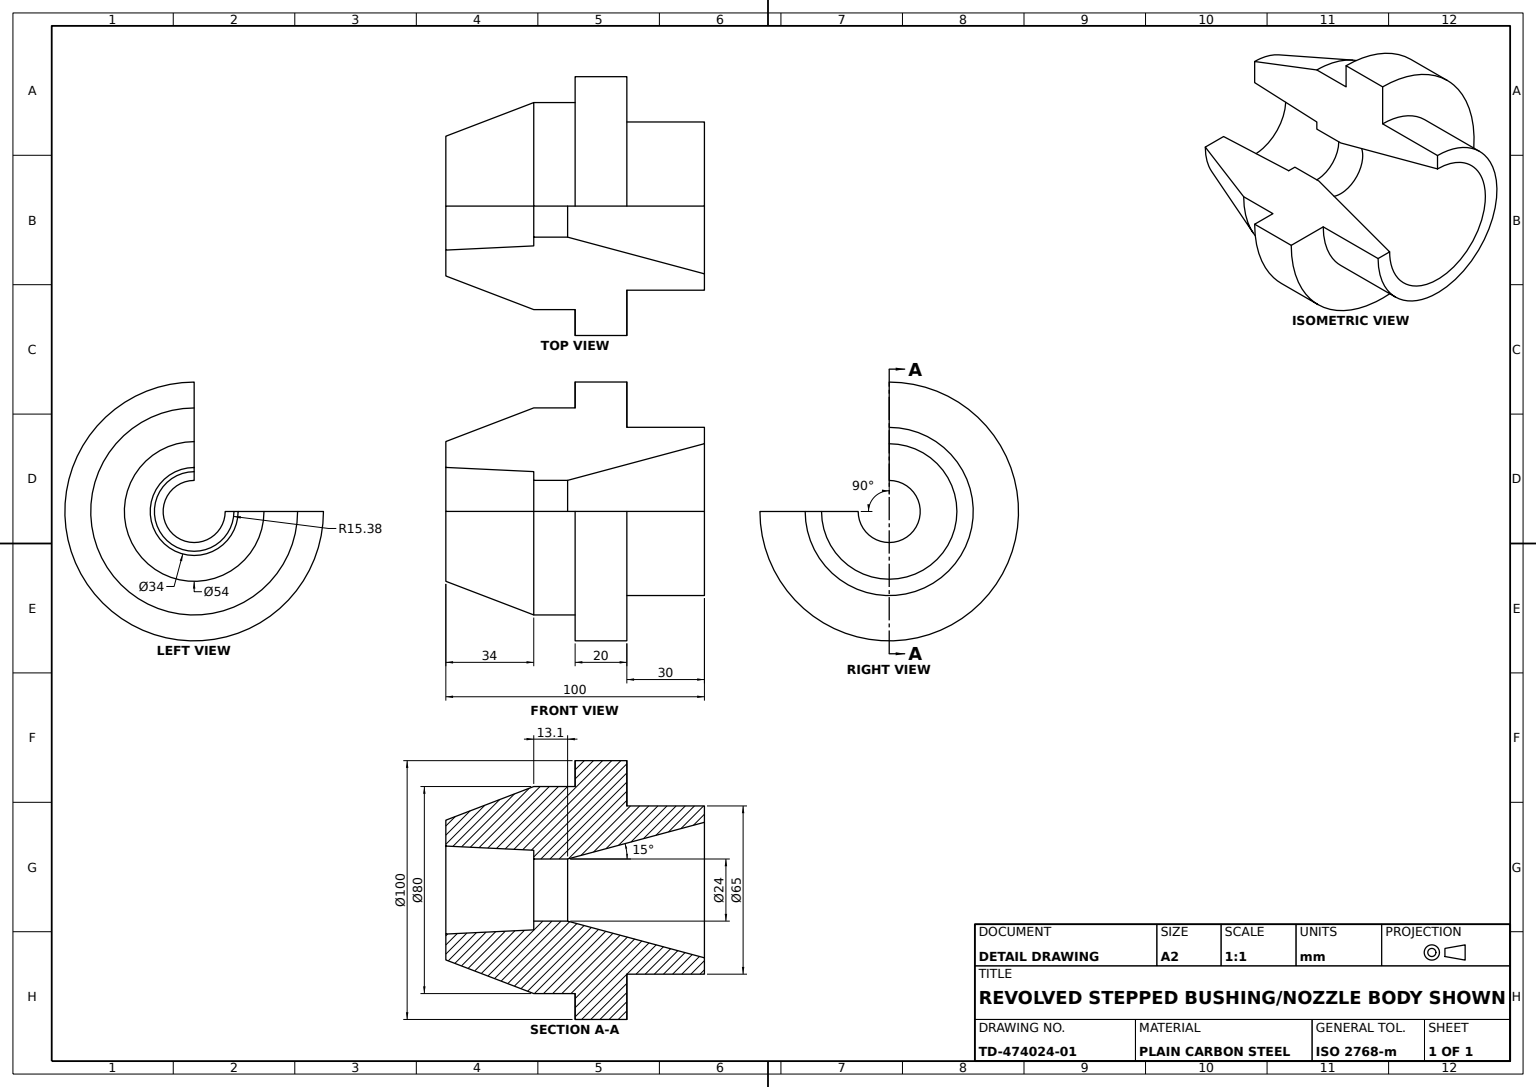
SolidWorks part; units mm, degrees
material "Plain Carbon Steel"
ref_plane "Front Plane" through (0, 0, 0) normal (0, 0, 1) x (1, 0, 0)
ref_plane "Top Plane" through (0, 0, 0) normal (0, 1, 0) x (1, 0, 0)
ref_plane "Right Plane" through (0, 0, 0) normal (1, 0, 0) x (0, 0, -1)
sketch "Hub Profile Sketch" plane through (0, 0, 0) normal (1, 0, 0) x (0, 0, -1)
  line L0 (0, 0) -> (0, 27)
  line L1 (0, 27) -> (34, 40)
  line L2 (34, 40) -> (50, 40)
  line L3 (50, 40) -> (50, 50)
  line L4 (50, 50) -> (70, 50)
  line L5 (70, 50) -> (70, 32.5)
  line L6 (70, 32.5) -> (100, 32.5)
  line L7 (100, 32.5) -> (100, 0)
  line L8 (100, 0) -> (0, 0)
  dimension "D1" = 32.5
  dimension "D2" = 50
  dimension "D3" = 40
  dimension "D4" = 27
  dimension "D5" = 34
  dimension "D6" = 20
  dimension "D7" = 30
  dimension "D8" = 100
revolve "Hub Body Revolve 270deg" add sketch "Hub Profile Sketch" angle 270 about L8
sketch "Tapered Bore Profile Sketch" plane through (0, 0, 0) normal (1, 0, 0) x (0, 0, -1)
  line L0 (0, 0) -> (0, 17)
  line L1 (0, 0) -> (100, 0)
  line L2 (100, 0) -> (100, 26.1756)
  line L3 (100, 26.1756) -> (47.0958, 12)
  line L4 (47.0958, 12) -> (34, 12)
  line L5 (34, 12) -> (34, 15.38)
  line L6 (0, 17) -> (34, 15.38)
  line L7 (100, 0) -> (100, 32.5) construction
  dimension "D1" = 15
  dimension "D2" = 13.0958
  dimension "D3" = 34
  dimension "D4" = 17
  dimension "D5" = 12
  dimension "D6" = 15.38
revolve "Stepped Tapered Bore Cut" cut sketch "Tapered Bore Profile Sketch" angle 360 about L1
